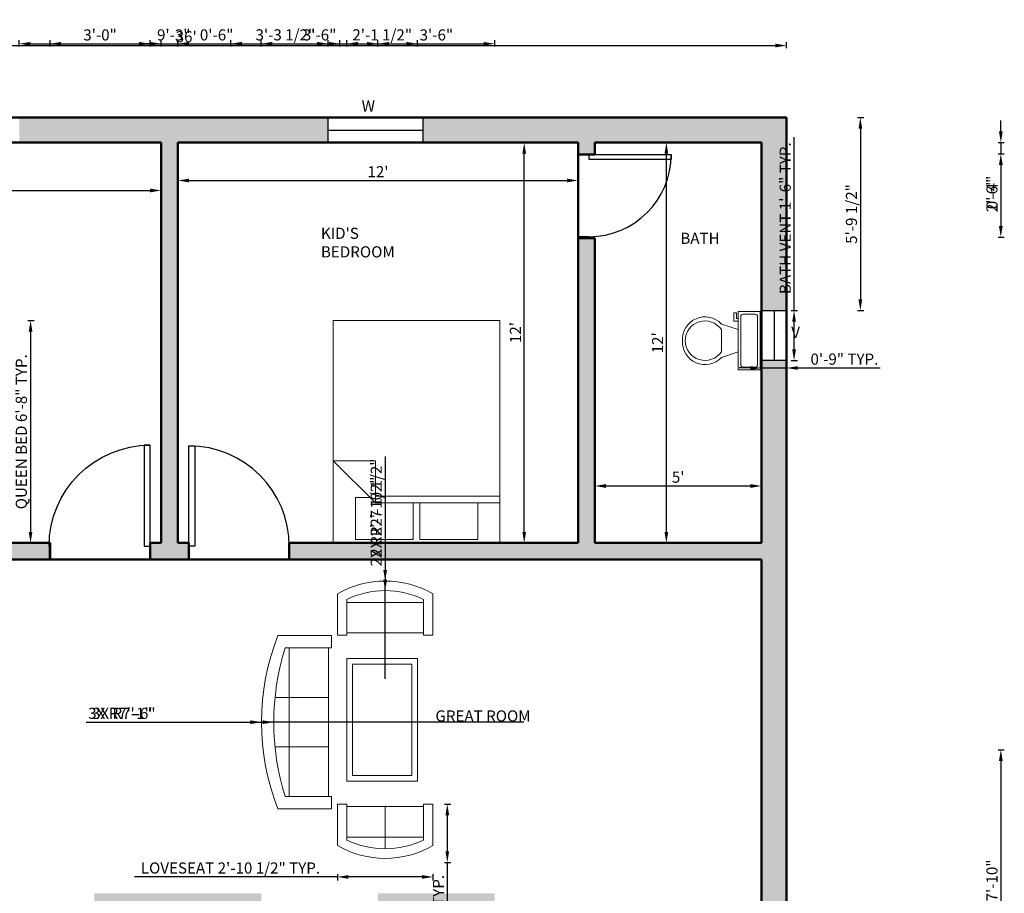
# Model space of a CAD drawing. Units: inches. Extents: x -31 to 511, y -453 to 49.
# Tile 4 of 4: x 157 to 511, y -265 to 49. Entities that reach past the tile are written whole.
import ezdxf

# ---------------------------------------------------------------- set-up
doc = ezdxf.new("R2010")
doc.units = ezdxf.units.IN
for name, color, linetype, lineweight in [('A-ANNO-DIMS', 2, 'Continuous', 18), ('A-ANNO-TEXT', 7, 'Continuous', 18), ('A-AREA-IDEN', 7, 'Continuous', 25), ('A-DOOR', 3, 'Continuous', 25), ('A-FLOR-FIXT', 9, 'Continuous', 18), ('A-FURN', 8, 'Continuous', 18), ('A-GLAZ', 4, 'Continuous', 25), ('A-WALL', 7, 'Continuous', 50), ('A-WALL-PATT', 252, 'Continuous', 13)]:
    doc.layers.add(name, color=color, linetype=linetype, lineweight=lineweight)
doc.styles.get("Standard").update_dxf_attribs({"font": 'arial.ttf'})
doc.dimstyles.new('ISO-25', dxfattribs={"dimtxt": 4, "dimasz": 4, "dimexe": 1.25, "dimexo": 0.625, "dimtad": 1, "dimlunit": 3, "dimtxsty": 'Standard', "dimcen": 2.5, "dimadec": 0, "dimazin": 0, "dimtfac": 1, "dimtmove": 0, "dimatfit": 3, "dimfxl": 1, "dimfxlon": 1, "dimarcsym": 0})

# ---------------------------------------------------------------- blocks, each defined once
blk = doc.blocks.new('*U2')
for p, q in [((0, 0), (0, -100)), ((750, 0), (750, -100))]:
    blk.add_line(p, q)
blk.add_lwpolyline([(0, 0), (0, 750), (43.75, 750), (43.75, 0)], close=True)
blk.add_arc((0, 0), 750, 0, 90)
blk = doc.blocks.new('*U4')
for p, q in [((9.5, -6), (9.5, -2)), ((-10, -8.5), (-8, -8.5)), ((-10, -9.5), (-10, -8.5)), ((-7, -9.5), (-10, -9.5)), ((-8, -8.5), (-8, -8)), ((-7, -8), (-7, -9.5)), ((-4, -8), (-6, -14)), ((4, -8), (6, -14)), ((4, -14), (-4, -14))]:
    blk.add_line(p, q)
blk.add_lwpolyline([(10.5, -8), (10.5, 0), (-10.5, 0), (-10.5, -8)], close=True)
for points in [[(-9.5, -2), (-9.5, -6)], [(8.5, -1), (-8.5, -1)], [(-8.5, -7), (8.5, -7)]]:
    blk.add_lwpolyline(points)
for centre, radius, start, end in [((-8.625, -1.875), 0.8839, 81.8699, 188.1301), ((8.625, -1.875), 0.8839, 351.8699, 98.1301), ((-8.625, -6.125), 0.8839, 171.869898, 278.1301), ((8.625, -6.125), 0.8839, 261.8699, 8.1301), ((-0.4772, -19.9188), 8.0953, 133.01722, 273.38), ((0.0374, -19.8731), 7.127, 124.50543, 269.7), ((-0.0373, -19.8731), 7.127, 270.3, 55.4946), ((0.4773, -19.9188), 8.0953, 266.62, 46.9828)]:
    blk.add_arc(centre, radius, start, end)
blk = doc.blocks.new('Sofa - Roundback Loveseat 5 ft.')
for p, q in [((0, -32.44198), (0, -5.99998)), ((-24, -33.99998), (-24, -11.46958)), ((24.00004, -33.99998), (24.00004, -11.46958)), ((-23.9998, -13.38178), (23.99986, -13.38178)), ((-24, -32.44198), (24.00004, -32.44198))]:
    blk.add_line(p, q)
for points in [[(-24, -33.99998), (-30, -33.99998), (-30, -7.99998)], [(30.00004, -7.99998), (30.00004, -33.99998), (24.00004, -33.99998)]]:
    blk.add_lwpolyline(points)
for centre, radius, start, end in [((0, -60.24998), 60.24998, 60.13715, 119.8628), ((0, -61.38438), 55.38444, 64.32083, 115.6792)]:
    blk.add_arc(centre, radius, start, end)
blk = doc.blocks.new('Bed - Queen')
for p, q in [((0, -80.00003), (0, 0)), ((0, 0), (59.99999, 0)), ((59.99999, 0), (59.99999, -80.00003)), ((7.99999, -1.2), (28.79998, -1.2)), ((7.99999, -14.4), (7.99999, -1.2)), ((28.79998, -1.2), (28.79998, -14.4)), ((31.19999, -1.2), (51.99999, -1.2)), ((31.19999, -14.4), (31.19999, -1.2)), ((51.99999, -1.2), (51.99999, -16.4)), ((0, -14.4), (44.8, -14.4)), ((44.8, -16.8), (0, -16.8)), ((59.99999, -29.6), (44.8, -14.4)), ((44.8, -14.4), (44.8, -29.6)), ((51.99999, -16.4), (46.79936, -16.4)), ((44.8, -29.6), (59.99999, -29.6)), ((59.99999, -80.00003), (0, -80.00003))]:
    blk.add_line(p, q)
blk = doc.blocks.new('Sofa - Roundback 7 ft.')
for p, q in [((-12.00002, -32.4421), (-12.00003, -6.5971)), ((11.99997, -32.4421), (11.99998, -6.5971)), ((-36.000027, -34), (-36.000027, -11.4696)), ((-35.999844, -13.3819), (35.9998, -13.3819)), ((35.99998, -34), (35.99998, -11.4696)), ((-36.000027, -32.4421), (35.99998, -32.4421))]:
    blk.add_line(p, q)
for points in [[(-36.000027, -34), (-42.000027, -34), (-42.000027, -8)], [(41.99998, -8), (41.99998, -34), (35.99998, -34)]]:
    blk.add_lwpolyline(points)
for centre, radius, start, end in [((0, -114.25), 114.25, 68.43141, 111.5686), ((-0.00001, -127.1968), 121.1968, 72.72033, 107.2797)]:
    blk.add_arc(centre, radius, start, end)
blk = doc.blocks.new('*D14')
at = {"layer": 'A-ANNO-DIMS', "color": 0, "lineweight": -2, "transparency": 16777216}
for p, q in [((63.46, -11.59), (63.46, -13.84)), ((67.46, -12.59), (203.46, -12.59)), ((207.46, -11.59), (207.46, -13.84))]:
    blk.add_line(p, q, dxfattribs=at)
at = {"layer": 'A-ANNO-DIMS', "color": 0, "transparency": 16777216}
for points in [[(67.46, -11.92), (67.46, -13.25), (63.46, -12.59)], [(203.46, -11.92), (203.46, -13.25), (207.46, -12.59)]]:
    blk.add_solid(points, dxfattribs=at)
at = {"layer": 'Defpoints', "color": 0, "transparency": 16777216}
for p in [(63.46, 4.62), (207.46, 4.62), (207.46, -12.59)]:
    blk.add_point(p, dxfattribs=at)
at = {"layer": 'A-ANNO-DIMS', "color": 0, "transparency": 16777216, "insert": (135.46, -9.95), "char_height": 4, "attachment_point": 5}
blk.add_mtext("12'", dxfattribs=at)
blk = doc.blocks.new('*D16')
at = {"layer": 'A-ANNO-DIMS', "color": 0, "lineweight": -2, "transparency": 16777216}
for p, q in [((213.46, -8.01), (213.46, -10.26)), ((217.46, -9.01), (353.46, -9.01)), ((357.46, -8.01), (357.46, -10.26))]:
    blk.add_line(p, q, dxfattribs=at)
at = {"layer": 'A-ANNO-DIMS', "color": 0, "transparency": 16777216}
for points in [[(217.46, -8.34), (217.46, -9.67), (213.46, -9.01)], [(353.46, -8.34), (353.46, -9.67), (357.46, -9.01)]]:
    blk.add_solid(points, dxfattribs=at)
at = {"layer": 'Defpoints', "color": 0, "transparency": 16777216}
for p in [(213.46, 4.62), (357.46, 4.62), (357.46, -9.01)]:
    blk.add_point(p, dxfattribs=at)
at = {"layer": 'A-ANNO-DIMS', "color": 0, "transparency": 16777216, "insert": (285.46, -6.37), "char_height": 4, "attachment_point": 5}
blk.add_mtext("12'", dxfattribs=at)
blk = doc.blocks.new('*D17')
at = {"layer": 'A-ANNO-DIMS', "color": 0, "lineweight": -2, "transparency": 16777216}
for p, q in [((339.07, 4.62), (336.82, 4.62)), ((338.07, -135.38), (338.07, 0.62)), ((339.07, -139.38), (336.82, -139.38))]:
    blk.add_line(p, q, dxfattribs=at)
at = {"layer": 'A-ANNO-DIMS', "color": 0, "transparency": 16777216}
for points in [[(337.4, 0.62), (338.73, 0.62), (338.07, 4.62)], [(337.4, -135.38), (338.73, -135.38), (338.07, -139.38)]]:
    blk.add_solid(points, dxfattribs=at)
at = {"layer": 'Defpoints', "color": 0, "transparency": 16777216}
for p in [(338.07, 4.62), (357.46, 4.62), (357.46, -139.38)]:
    blk.add_point(p, dxfattribs=at)
at = {"layer": 'A-ANNO-DIMS', "color": 0, "transparency": 16777216, "insert": (335.43, -63.69), "char_height": 4, "attachment_point": 5, "rotation": 90}
blk.add_mtext("12'", dxfattribs=at)
blk = doc.blocks.new('*D18')
at = {"layer": 'A-ANNO-DIMS', "color": 0, "lineweight": -2, "transparency": 16777216}
for p, q in [((363.46, -119.88), (363.46, -117.63)), ((367.46, -118.88), (419.46, -118.88)), ((423.46, -119.88), (423.46, -117.63))]:
    blk.add_line(p, q, dxfattribs=at)
at = {"layer": 'A-ANNO-DIMS', "color": 0, "transparency": 16777216}
for points in [[(367.46, -118.21), (367.46, -119.55), (363.46, -118.88)], [(419.46, -118.21), (419.46, -119.55), (423.46, -118.88)]]:
    blk.add_solid(points, dxfattribs=at)
at = {"layer": 'Defpoints', "color": 0, "transparency": 16777216}
for p in [(423.46, -118.88), (363.46, -139.38), (423.46, -139.38)]:
    blk.add_point(p, dxfattribs=at)
at = {"layer": 'A-ANNO-DIMS', "color": 0, "transparency": 16777216, "insert": (393.46, -116.22), "char_height": 4, "attachment_point": 5}
blk.add_mtext("5'", dxfattribs=at)
blk = doc.blocks.new('*D19')
at = {"layer": 'A-ANNO-DIMS', "color": 0, "lineweight": -2, "transparency": 16777216}
for p, q in [((390.21, 4.62), (387.96, 4.62)), ((389.21, -135.38), (389.21, 0.62)), ((390.21, -139.38), (387.96, -139.38))]:
    blk.add_line(p, q, dxfattribs=at)
at = {"layer": 'A-ANNO-DIMS', "color": 0, "transparency": 16777216}
for points in [[(388.54, 0.62), (389.88, 0.62), (389.21, 4.62)], [(388.54, -135.38), (389.88, -135.38), (389.21, -139.38)]]:
    blk.add_solid(points, dxfattribs=at)
at = {"layer": 'Defpoints', "color": 0, "transparency": 16777216}
for p in [(389.21, 4.62), (423.46, 4.62), (423.46, -139.38)]:
    blk.add_point(p, dxfattribs=at)
at = {"layer": 'A-ANNO-DIMS', "color": 0, "transparency": 16777216, "insert": (386.58, -67.38), "char_height": 4, "attachment_point": 5, "rotation": 90}
blk.add_mtext("12'", dxfattribs=at)
blk = doc.blocks.new('*D26')
at = {"layer": 'A-ANNO-DIMS', "color": 0, "lineweight": -2, "transparency": 16777216}
for p, q in [((0.46, 38.54), (0.46, 40.79)), ((4.46, 39.54), (428.46, 39.54)), ((432.46, 38.54), (432.46, 40.79))]:
    blk.add_line(p, q, dxfattribs=at)
at = {"layer": 'A-ANNO-DIMS', "color": 0, "transparency": 16777216}
for points in [[(4.46, 40.2), (4.46, 38.87), (0.46, 39.54)], [(428.46, 40.2), (428.46, 38.87), (432.46, 39.54)]]:
    blk.add_solid(points, dxfattribs=at)
at = {"layer": 'Defpoints', "color": 0, "transparency": 16777216}
for p in [(432.46, 39.54), (0.46, 13.62), (432.46, 13.62)]:
    blk.add_point(p, dxfattribs=at)
at = {"layer": 'A-ANNO-DIMS', "color": 0, "transparency": 16777216, "insert": (216.46, 42.21), "char_height": 4, "attachment_point": 5}
blk.add_mtext("36'", dxfattribs=at)
blk = doc.blocks.new('WIN-34IN')
blk.add_line((0, 4.5), (34, 4.5))
blk.add_lwpolyline([(0, 9), (34, 9), (34, 0), (0, 0)], close=True)
blk = doc.blocks.new('VENT-18IN')
blk.add_line((4.5, 18), (4.5, 0))
blk.add_lwpolyline([(0, 18), (9, 18), (9, 0), (0, 0)], close=True)
blk = doc.blocks.new('*D32')
at = {"layer": 'A-ANNO-DIMS', "color": 0, "lineweight": -2, "transparency": 16777216}
for p, q in [((435.16, -55.74), (435.16, 6.62)), ((434.16, -55.74), (436.41, -55.74)), ((435.16, -69.74), (435.16, -59.74)), ((434.16, -73.74), (436.41, -73.74))]:
    blk.add_line(p, q, dxfattribs=at)
at = {"layer": 'A-ANNO-DIMS', "color": 0, "transparency": 16777216}
for points in [[(434.5, -59.74), (435.83, -59.74), (435.16, -55.74)], [(434.5, -69.74), (435.83, -69.74), (435.16, -73.74)]]:
    blk.add_solid(points, dxfattribs=at)
at = {"layer": 'Defpoints', "color": 0, "transparency": 16777216}
for p in [(432.46, -55.74), (435.16, -55.74), (432.46, -73.74)]:
    blk.add_point(p, dxfattribs=at)
at = {"layer": 'A-ANNO-DIMS', "color": 0, "transparency": 16777216, "insert": (432.5, -22.56), "char_height": 4, "attachment_point": 5, "rotation": 90}
blk.add_mtext('BATH VENT 1\'-6" TYP.', dxfattribs=at)
blk = doc.blocks.new('*D33')
at = {"layer": 'A-ANNO-DIMS', "color": 0, "lineweight": -2, "transparency": 16777216}
for p, q in [((419.46, -76.44), (415.46, -76.44)), ((423.46, -75.44), (423.46, -77.69)), ((423.46, -76.44), (432.46, -76.44)), ((432.46, -75.44), (432.46, -77.69)), ((436.46, -76.44), (466.1, -76.44))]:
    blk.add_line(p, q, dxfattribs=at)
at = {"layer": 'A-ANNO-DIMS', "color": 0, "transparency": 16777216}
for points in [[(419.46, -75.78), (419.46, -77.11), (423.46, -76.44)], [(436.46, -75.78), (436.46, -77.11), (432.46, -76.44)]]:
    blk.add_solid(points, dxfattribs=at)
at = {"layer": 'Defpoints', "color": 0, "transparency": 16777216}
for p in [(423.46, -73.74), (432.46, -73.74), (432.46, -76.44)]:
    blk.add_point(p, dxfattribs=at)
at = {"layer": 'A-ANNO-DIMS', "color": 0, "transparency": 16777216, "insert": (453.28, -73.77), "char_height": 4, "attachment_point": 5}
blk.add_mtext('0\'-9" TYP.', dxfattribs=at)
blk = doc.blocks.new('*D34')
at = {"layer": 'A-ANNO-DIMS', "color": 0, "lineweight": -2, "transparency": 16777216}
for p, q in [((159.47, -59.38), (161.72, -59.38)), ((160.47, -63.38), (160.47, -135.38)), ((159.47, -139.38), (161.72, -139.38))]:
    blk.add_line(p, q, dxfattribs=at)
at = {"layer": 'A-ANNO-DIMS', "color": 0, "transparency": 16777216}
for points in [[(159.8, -63.38), (161.13, -63.38), (160.47, -59.38)], [(159.8, -135.38), (161.13, -135.38), (160.47, -139.38)]]:
    blk.add_solid(points, dxfattribs=at)
at = {"layer": 'Defpoints', "color": 0, "transparency": 16777216}
for p in [(148.47, -59.38), (148.47, -139.38), (160.47, -139.38)]:
    blk.add_point(p, dxfattribs=at)
at = {"layer": 'A-ANNO-DIMS', "color": 0, "transparency": 16777216, "insert": (157.65, -99.38), "char_height": 4, "attachment_point": 5, "rotation": 90}
blk.add_mtext('QUEEN BED 6\'-8" TYP.', dxfattribs=at)
blk = doc.blocks.new('*D38')
at = {"layer": 'A-ANNO-DIMS', "color": 0, "lineweight": -2, "transparency": 16777216}
for p, q in [((270.85, -258.5), (270.85, -260.75)), ((305.24, -258.5), (305.24, -260.75)), ((270.85, -259.5), (197.91, -259.5)), ((301.24, -259.5), (274.85, -259.5))]:
    blk.add_line(p, q, dxfattribs=at)
at = {"layer": 'A-ANNO-DIMS', "color": 0, "transparency": 16777216}
for points in [[(274.85, -258.83), (274.85, -260.17), (270.85, -259.5)], [(301.24, -258.83), (301.24, -260.17), (305.24, -259.5)]]:
    blk.add_solid(points, dxfattribs=at)
at = {"layer": 'Defpoints', "color": 0, "transparency": 16777216}
for p in [(270.85, -254.34), (305.24, -254.34), (270.85, -259.5)]:
    blk.add_point(p, dxfattribs=at)
at = {"layer": 'A-ANNO-DIMS', "color": 0, "transparency": 16777216, "insert": (232.38, -256.8), "char_height": 4, "attachment_point": 5}
blk.add_mtext('LOVESEAT 2\'-10 1/2" TYP.', dxfattribs=at)
blk = doc.blocks.new('*D39')
at = {"layer": 'A-ANNO-DIMS', "color": 0, "lineweight": -2, "transparency": 16777216}
for p, q in [((309.4, -233.32), (311.65, -233.32)), ((310.4, -237.32), (310.4, -250.34)), ((309.4, -254.34), (311.65, -254.34)), ((310.4, -254.34), (310.4, -283.6))]:
    blk.add_line(p, q, dxfattribs=at)
at = {"layer": 'A-ANNO-DIMS', "color": 0, "transparency": 16777216}
for points in [[(309.73, -237.32), (311.06, -237.32), (310.4, -233.32)], [(309.73, -250.34), (311.06, -250.34), (310.4, -254.34)]]:
    blk.add_solid(points, dxfattribs=at)
at = {"layer": 'Defpoints', "color": 0, "transparency": 16777216}
for p in [(305.24, -233.32), (305.24, -254.34), (310.4, -254.34)]:
    blk.add_point(p, dxfattribs=at)
at = {"layer": 'A-ANNO-DIMS', "color": 0, "transparency": 16777216, "insert": (307.73, -270.97), "char_height": 4, "attachment_point": 5, "rotation": 90}
blk.add_mtext('1\'-9" TYP.', dxfattribs=at)
blk = doc.blocks.new('*D50')
at = {"layer": 'A-ANNO-DIMS', "color": 0, "lineweight": -2, "transparency": 16777216}
for p, q in [((167.46, 39.17), (167.46, 41.42)), ((171.46, 40.17), (199.46, 40.17)), ((203.46, 39.17), (203.46, 41.42))]:
    blk.add_line(p, q, dxfattribs=at)
at = {"layer": 'A-ANNO-DIMS', "color": 0, "transparency": 16777216}
for points in [[(171.46, 40.84), (171.46, 39.5), (167.46, 40.17)], [(199.46, 40.84), (199.46, 39.5), (203.46, 40.17)]]:
    blk.add_solid(points, dxfattribs=at)
at = {"layer": 'Defpoints', "color": 0, "transparency": 16777216}
for p in [(203.46, 40.17), (167.46, -139.38), (203.46, -139.38)]:
    blk.add_point(p, dxfattribs=at)
at = {"layer": 'A-ANNO-DIMS', "color": 0, "transparency": 16777216, "insert": (185.46, 42.84), "char_height": 4, "attachment_point": 5}
blk.add_mtext('3\'-0"', dxfattribs=at)
blk = doc.blocks.new('*D51')
at = {"layer": 'A-ANNO-DIMS', "color": 0, "lineweight": -2, "transparency": 16777216}
for p, q in [((508.55, 0.62), (510.8, 0.62)), ((509.55, -3.38), (509.55, -25.38)), ((508.55, -29.38), (510.8, -29.38))]:
    blk.add_line(p, q, dxfattribs=at)
at = {"layer": 'A-ANNO-DIMS', "color": 0, "transparency": 16777216}
for points in [[(508.88, -3.38), (510.22, -3.38), (509.55, 0.62)], [(508.88, -25.38), (510.22, -25.38), (509.55, -29.38)]]:
    blk.add_solid(points, dxfattribs=at)
at = {"layer": 'Defpoints', "color": 0, "transparency": 16777216}
for p in [(57.46, 0.62), (57.46, -29.38), (509.55, -29.38)]:
    blk.add_point(p, dxfattribs=at)
at = {"layer": 'A-ANNO-DIMS', "color": 0, "transparency": 16777216, "insert": (506.88, -14.38), "char_height": 4, "attachment_point": 5, "rotation": 90}
blk.add_mtext('2\'-6"', dxfattribs=at)
blk = doc.blocks.new('*D52')
at = {"layer": 'A-ANNO-DIMS', "color": 0, "lineweight": -2, "transparency": 16777216}
for p, q in [((243.45, 39.17), (243.45, 41.42)), ((247.45, 40.17), (281.45, 40.17)), ((285.45, 39.17), (285.45, 41.42))]:
    blk.add_line(p, q, dxfattribs=at)
at = {"layer": 'A-ANNO-DIMS', "color": 0, "transparency": 16777216}
for points in [[(247.45, 40.84), (247.45, 39.5), (243.45, 40.17)], [(281.45, 40.84), (281.45, 39.5), (285.45, 40.17)]]:
    blk.add_solid(points, dxfattribs=at)
at = {"layer": 'Defpoints', "color": 0, "transparency": 16777216}
for p in [(285.45, 40.17), (243.45, -265.38), (285.45, -265.38)]:
    blk.add_point(p, dxfattribs=at)
at = {"layer": 'A-ANNO-DIMS', "color": 0, "transparency": 16777216, "insert": (264.45, 42.84), "char_height": 4, "attachment_point": 5}
blk.add_mtext('3\'-6"', dxfattribs=at)
blk = doc.blocks.new('*D53')
at = {"layer": 'A-ANNO-DIMS', "color": 0, "lineweight": -2, "transparency": 16777216}
for p, q in [((203.46, 40.17), (199.46, 40.17)), ((207.46, 39.17), (207.46, 41.42)), ((207.46, 40.17), (213.46, 40.17)), ((213.46, 39.17), (213.46, 41.42)), ((217.46, 40.17), (233.35, 40.17))]:
    blk.add_line(p, q, dxfattribs=at)
at = {"layer": 'A-ANNO-DIMS', "color": 0, "transparency": 16777216}
for points in [[(203.46, 40.84), (203.46, 39.5), (207.46, 40.17)], [(217.46, 40.84), (217.46, 39.5), (213.46, 40.17)]]:
    blk.add_solid(points, dxfattribs=at)
at = {"layer": 'Defpoints', "color": 0, "transparency": 16777216}
for p in [(213.46, 40.17), (207.46, 4.62), (213.46, 4.62)]:
    blk.add_point(p, dxfattribs=at)
at = {"layer": 'A-ANNO-DIMS', "color": 0, "transparency": 16777216, "insert": (227.41, 42.84), "char_height": 4, "attachment_point": 5}
blk.add_mtext('0\'-6"', dxfattribs=at)
blk = doc.blocks.new('*D55')
at = {"layer": 'A-ANNO-DIMS', "color": 0, "lineweight": -2, "transparency": 16777216}
for p, q in [((156.41, 39.17), (156.41, 41.42)), ((160.41, 40.17), (263.57, 40.17)), ((267.57, 39.17), (267.57, 41.42))]:
    blk.add_line(p, q, dxfattribs=at)
at = {"layer": 'A-ANNO-DIMS', "color": 0, "transparency": 16777216}
for points in [[(160.41, 40.84), (160.41, 39.5), (156.41, 40.17)], [(263.57, 40.84), (263.57, 39.5), (267.57, 40.17)]]:
    blk.add_solid(points, dxfattribs=at)
at = {"layer": 'Defpoints', "color": 0, "transparency": 16777216}
for p in [(267.57, 40.17), (156.41, 13.62), (267.57, 13.62)]:
    blk.add_point(p, dxfattribs=at)
at = {"layer": 'A-ANNO-DIMS', "color": 0, "transparency": 16777216, "insert": (211.99, 42.84), "char_height": 4, "attachment_point": 5}
blk.add_mtext('9\'-3"', dxfattribs=at)
blk = doc.blocks.new('*D56')
at = {"layer": 'A-ANNO-DIMS', "color": 0, "lineweight": -2, "transparency": 16777216}
for p, q in [((458.01, 13.62), (460.26, 13.62)), ((459.01, 9.62), (459.01, -51.74)), ((458.01, -55.74), (460.26, -55.74))]:
    blk.add_line(p, q, dxfattribs=at)
at = {"layer": 'A-ANNO-DIMS', "color": 0, "transparency": 16777216}
for points in [[(458.35, 9.62), (459.68, 9.62), (459.01, 13.62)], [(458.35, -51.74), (459.68, -51.74), (459.01, -55.74)]]:
    blk.add_solid(points, dxfattribs=at)
at = {"layer": 'Defpoints', "color": 0, "transparency": 16777216}
for p in [(432.46, 13.62), (432.46, -55.74), (459.01, -55.74)]:
    blk.add_point(p, dxfattribs=at)
at = {"layer": 'A-ANNO-DIMS', "color": 0, "transparency": 16777216, "insert": (456.32, -21.06), "char_height": 4, "attachment_point": 5, "rotation": 90}
blk.add_mtext('5\'-9 1/2"', dxfattribs=at)
blk = doc.blocks.new('*D58')
at = {"layer": 'A-ANNO-DIMS', "color": 0, "lineweight": -2, "transparency": 16777216}
for p, q in [((508.55, -213.76), (510.8, -213.76)), ((509.55, -217.76), (509.55, -303.74)), ((508.55, -307.74), (510.8, -307.74))]:
    blk.add_line(p, q, dxfattribs=at)
at = {"layer": 'A-ANNO-DIMS', "color": 0, "transparency": 16777216}
for points in [[(508.88, -217.76), (510.22, -217.76), (509.55, -213.76)], [(508.88, -303.74), (510.22, -303.74), (509.55, -307.74)]]:
    blk.add_solid(points, dxfattribs=at)
at = {"layer": 'Defpoints', "color": 0, "transparency": 16777216}
for p in [(9.46, -213.76), (9.46, -307.74), (509.55, -307.74)]:
    blk.add_point(p, dxfattribs=at)
at = {"layer": 'A-ANNO-DIMS', "color": 0, "transparency": 16777216, "insert": (506.88, -260.75), "char_height": 4, "attachment_point": 5, "rotation": 90}
blk.add_mtext('7\'-10"', dxfattribs=at)
blk = doc.blocks.new('*D63')
at = {"layer": 'A-ANNO-DIMS', "color": 0, "lineweight": -2, "transparency": 16777216}
for p, q in [((285.45, 39.17), (285.45, 41.42)), ((289.45, 40.17), (323.46, 40.17)), ((327.46, 39.17), (327.46, 41.42))]:
    blk.add_line(p, q, dxfattribs=at)
at = {"layer": 'A-ANNO-DIMS', "color": 0, "transparency": 16777216}
for points in [[(289.45, 40.84), (289.45, 39.5), (285.45, 40.17)], [(323.46, 40.84), (323.46, 39.5), (327.46, 40.17)]]:
    blk.add_solid(points, dxfattribs=at)
at = {"layer": 'Defpoints', "color": 0, "transparency": 16777216}
for p in [(327.46, 40.17), (285.45, -265.38), (327.46, -265.38)]:
    blk.add_point(p, dxfattribs=at)
at = {"layer": 'A-ANNO-DIMS', "color": 0, "transparency": 16777216, "insert": (306.46, 42.84), "char_height": 4, "attachment_point": 5}
blk.add_mtext('3\'-6"', dxfattribs=at)
blk = doc.blocks.new('*D67')
at = {"layer": 'A-ANNO-DIMS', "color": 0, "lineweight": -2, "transparency": 16777216}
for p, q in [((274.24, 39.17), (274.24, 41.42)), ((278.24, 40.17), (295.69, 40.17)), ((299.69, 39.17), (299.69, 41.42))]:
    blk.add_line(p, q, dxfattribs=at)
at = {"layer": 'A-ANNO-DIMS', "color": 0, "transparency": 16777216}
for points in [[(278.24, 40.84), (278.24, 39.5), (274.24, 40.17)], [(295.69, 40.84), (295.69, 39.5), (299.69, 40.17)]]:
    blk.add_solid(points, dxfattribs=at)
at = {"layer": 'Defpoints', "color": 0, "transparency": 16777216}
for p in [(299.69, 40.17), (274.24, -180.94), (299.69, -180.94)]:
    blk.add_point(p, dxfattribs=at)
at = {"layer": 'A-ANNO-DIMS', "color": 0, "transparency": 16777216, "insert": (286.97, 42.86), "char_height": 4, "attachment_point": 5}
blk.add_mtext('2\'-1 1/2"', dxfattribs=at)
blk = doc.blocks.new('*D68')
at = {"layer": 'A-ANNO-DIMS', "color": 0, "lineweight": -2, "transparency": 16777216}
for p, q in [((-25.09, -180.94), (-27.34, -180.94)), ((-26.09, -221.03), (-26.09, -184.94)), ((-25.09, -225.03), (-27.34, -225.03))]:
    blk.add_line(p, q, dxfattribs=at)
at = {"layer": 'A-ANNO-DIMS', "color": 0, "transparency": 16777216}
for points in [[(-26.75, -184.94), (-25.42, -184.94), (-26.09, -180.94)], [(-26.75, -221.03), (-25.42, -221.03), (-26.09, -225.03)]]:
    blk.add_solid(points, dxfattribs=at)
at = {"layer": 'Defpoints', "color": 0, "transparency": 16777216}
for p in [(-26.09, -180.94), (299.69, -180.94), (299.69, -225.03)]:
    blk.add_point(p, dxfattribs=at)
at = {"layer": 'A-ANNO-DIMS', "color": 0, "transparency": 16777216, "insert": (-28.75, -202.99), "char_height": 4, "attachment_point": 5, "rotation": 90}
blk.add_mtext('3\'-8"', dxfattribs=at)
blk = doc.blocks.new('*D69')
at = {"layer": 'A-ANNO-DIMS', "color": 0, "lineweight": -2, "transparency": 16777216}
for p, q in [((232.48, 39.17), (232.48, 41.42)), ((236.48, 40.17), (267.79, 40.17)), ((271.79, 39.17), (271.79, 41.42))]:
    blk.add_line(p, q, dxfattribs=at)
at = {"layer": 'A-ANNO-DIMS', "color": 0, "transparency": 16777216}
for points in [[(236.48, 40.84), (236.48, 39.5), (232.48, 40.17)], [(267.79, 40.84), (267.79, 39.5), (271.79, 40.17)]]:
    blk.add_solid(points, dxfattribs=at)
at = {"layer": 'Defpoints', "color": 0, "transparency": 16777216}
for p in [(271.79, 40.17), (232.48, -304.06), (271.79, -304.06)]:
    blk.add_point(p, dxfattribs=at)
at = {"layer": 'A-ANNO-DIMS', "color": 0, "transparency": 16777216, "insert": (252.13, 42.86), "char_height": 4, "attachment_point": 5}
blk.add_mtext('3\'-3 1/2"', dxfattribs=at)
blk = doc.blocks.new('*D71')
at = {"layer": 'A-ANNO-DIMS', "color": 0, "lineweight": -2, "transparency": 16777216}
for p, q in [((209.46, -444.93), (205.46, -444.93)), ((213.46, -443.93), (213.46, -446.18)), ((213.46, -444.93), (217.46, -444.93)), ((217.46, -443.93), (217.46, -446.18)), ((221.46, -444.93), (237.35, -444.93))]:
    blk.add_line(p, q, dxfattribs=at)
at = {"layer": 'A-ANNO-DIMS', "color": 0, "transparency": 16777216}
for points in [[(209.46, -444.26), (209.46, -445.6), (213.46, -444.93)], [(221.46, -444.26), (221.46, -445.6), (217.46, -444.93)]]:
    blk.add_solid(points, dxfattribs=at)
at = {"layer": 'Defpoints', "color": 0, "transparency": 16777216}
for p in [(213.46, -139.38), (217.46, -139.38), (217.46, -444.93)]:
    blk.add_point(p, dxfattribs=at)
at = {"layer": 'A-ANNO-DIMS', "color": 0, "transparency": 16777216, "insert": (231.41, -442.26), "char_height": 4, "attachment_point": 5}
blk.add_mtext('0\'-4"', dxfattribs=at)
blk = doc.blocks.new('*D72')
at = {"layer": 'A-ANNO-DIMS', "color": 0, "lineweight": -2, "transparency": 16777216}
for p, q in [((509.55, 8.62), (509.55, 12.62)), ((508.55, 4.62), (510.8, 4.62)), ((509.55, 4.62), (509.55, 0.62)), ((508.55, 0.62), (510.8, 0.62)), ((509.55, -3.38), (509.55, -19.26))]:
    blk.add_line(p, q, dxfattribs=at)
at = {"layer": 'A-ANNO-DIMS', "color": 0, "transparency": 16777216}
for points in [[(508.88, 8.62), (510.22, 8.62), (509.55, 4.62)], [(508.88, -3.38), (510.22, -3.38), (509.55, 0.62)]]:
    blk.add_solid(points, dxfattribs=at)
at = {"layer": 'Defpoints', "color": 0, "transparency": 16777216}
for p in [(57.46, 4.62), (57.46, 0.62), (509.55, 0.62)]:
    blk.add_point(p, dxfattribs=at)
at = {"layer": 'A-ANNO-DIMS', "color": 0, "transparency": 16777216, "insert": (506.88, -13.32), "char_height": 4, "attachment_point": 5, "rotation": 90}
blk.add_mtext('0\'-4"', dxfattribs=at)
blk = doc.blocks.new('*D73')
at = {"layer": 'A-ANNO-DIMS', "color": 0, "lineweight": -2, "transparency": 16777216}
for p, q in [((181.83, -203.84), (243.98, -203.84)), ((337.97, -203.84), (247.98, -203.84))]:
    blk.add_line(p, q, dxfattribs=at)
at = {"layer": 'A-ANNO-DIMS', "color": 0, "transparency": 16777216}
blk.add_solid([(243.98, -203.17), (243.98, -204.51), (247.98, -203.84)], dxfattribs=at)
at = {"layer": 'Defpoints', "color": 0, "transparency": 16777216}
for p in [(247.98, -203.84), (337.97, -203.84)]:
    blk.add_point(p, dxfattribs=at)
at = {"layer": 'A-ANNO-DIMS', "color": 0, "transparency": 16777216, "insert": (193.99, -201.17), "char_height": 4, "attachment_point": 5, "rotation": 359.9999}
blk.add_mtext('3X R7\'-6"', dxfattribs=at)
blk = doc.blocks.new('*D74')
at = {"layer": 'A-ANNO-DIMS', "color": 0, "lineweight": -2, "transparency": 16777216}
for p, q in [((180.47, -203.84), (239.52, -203.84)), ((328.36, -203.84), (243.52, -203.84))]:
    blk.add_line(p, q, dxfattribs=at)
at = {"layer": 'A-ANNO-DIMS', "color": 0, "transparency": 16777216}
blk.add_solid([(239.52, -203.17), (239.52, -204.51), (243.52, -203.84)], dxfattribs=at)
at = {"layer": 'Defpoints', "color": 0, "transparency": 16777216}
for p in [(243.52, -203.84), (328.36, -203.84)]:
    blk.add_point(p, dxfattribs=at)
at = {"layer": 'A-ANNO-DIMS', "color": 0, "transparency": 16777216, "insert": (192.63, -201.17), "char_height": 4, "attachment_point": 5, "rotation": 359.9999}
blk.add_mtext('3X R7\'-1"', dxfattribs=at)
blk = doc.blocks.new('*D75')
at = {"layer": 'A-ANNO-DIMS', "color": 0, "lineweight": -2, "transparency": 16777216}
for p, q in [((288.04, -108.28), (288.04, -149.08)), ((288.04, -187.61), (288.04, -153.08))]:
    blk.add_line(p, q, dxfattribs=at)
at = {"layer": 'A-ANNO-DIMS', "color": 0, "transparency": 16777216}
blk.add_solid([(287.38, -149.08), (288.71, -149.08), (288.04, -153.08)], dxfattribs=at)
at = {"layer": 'Defpoints', "color": 0, "transparency": 16777216}
for p in [(288.04, -153.08), (288.04, -187.61)]:
    blk.add_point(p, dxfattribs=at)
at = {"layer": 'A-ANNO-DIMS', "color": 0, "transparency": 16777216, "insert": (285.35, -126.68), "char_height": 4, "attachment_point": 5, "rotation": 89.9992}
blk.add_mtext('2X R2\'-10 1/2"', dxfattribs=at)
blk = doc.blocks.new('*D76')
at = {"layer": 'A-ANNO-DIMS', "color": 0, "lineweight": -2, "transparency": 16777216}
for p, q in [((288.04, -114.83), (288.04, -152.52)), ((288.04, -188.26), (288.04, -156.52))]:
    blk.add_line(p, q, dxfattribs=at)
at = {"layer": 'A-ANNO-DIMS', "color": 0, "transparency": 16777216}
blk.add_solid([(287.38, -152.52), (288.71, -152.52), (288.04, -156.52)], dxfattribs=at)
at = {"layer": 'Defpoints', "color": 0, "transparency": 16777216}
for p in [(288.04, -156.52), (288.04, -188.26)]:
    blk.add_point(p, dxfattribs=at)
at = {"layer": 'A-ANNO-DIMS', "color": 0, "transparency": 16777216, "insert": (285.35, -131.67), "char_height": 4, "attachment_point": 5, "rotation": 89.9991}
blk.add_mtext('2X R2\'-7 1/2"', dxfattribs=at)

msp = doc.modelspace()

# ---------------------------------------------------------------- hatches: boundary and pattern name
at = {"layer": 'A-WALL-PATT'}
h = msp.add_hatch(color=256, dxfattribs=at)
h.dxf.hatch_style = 1
h.paths.add_polyline_path([(122.408, 13.62), (0.465, 13.62), (0.465, -55.742), (9.465, -55.742), (9.465, 4.62), (57.465, 4.62), (57.465, 0.62), (59.528, 0.62), (63.465, 0.62), (63.465, 4.62), (122.408, 4.62)])
h.paths.add_polyline_path([(267.569, 13.62), (156.408, 13.62), (156.408, 4.62), (207.465, 4.62), (207.465, -139.38), (203.465, -139.38), (203.465, -140.534), (203.465, -145.38), (217.465, -145.38), (217.465, -140.567), (217.465, -139.38), (213.465, -139.38), (213.465, 4.62), (267.569, 4.62)])
h.paths.add_polyline_path([(432.465, 13.62), (301.569, 13.62), (301.569, 4.62), (357.465, 4.62), (357.465, 0.312), (361.402, 0.312), (363.465, 0.312), (363.465, 4.62), (423.465, 4.62), (423.465, -55.742), (432.465, -55.742)])
h.paths.add_polyline_path([(432.465, -73.742), (423.465, -73.742), (423.465, -139.38), (363.465, -139.38), (363.465, -29.688), (357.465, -29.688), (357.465, -139.38), (253.542, -139.38, -0.0082235), (253.561, -140.567), (253.561, -145.38), (423.465, -145.38), (423.465, -409.38), (414.601, -409.38), (414.601, -412.759), (414.601, -418.38), (432.465, -418.38)])
h.paths.add_polyline_path([(167.12, -140.534, -0.00794), (167.139, -139.38), (63.465, -139.38), (63.465, -29.38), (57.465, -29.38), (57.465, -57.083), (57.472, -57.083), (57.472, -78.083), (57.465, -139.38), (9.465, -139.38), (9.465, -73.742), (0.465, -73.742), (0.465, -179.759), (9.465, -179.759), (9.465, -145.38), (167.12, -145.38)])
h.paths.add_polyline_path([(372.446, -412.759, -0.0200643), (372.581, -409.38), (327.465, -409.38), (327.465, -265.38), (285.454, -265.38), (285.454, -271.38), (321.465, -271.38), (321.465, -409.38), (273.096, -409.38), (273.096, -418.38), (372.446, -418.38)], flags=17)
h.paths.add_polyline_path([(239.096, -409.38), (189.465, -409.38), (189.465, -271.38), (243.454, -271.38), (243.454, -265.38), (183.465, -265.38), (183.465, -409.38), (156.552, -409.38), (156.552, -418.38), (239.096, -418.38)])
h.paths.add_polyline_path([(122.552, -409.38), (111.465, -409.38), (111.465, -325.38), (105.465, -325.38), (105.465, -409.38), (72.938, -409.38), (72.938, -418.38), (122.552, -418.38)])
h.paths.add_polyline_path([(38.938, -409.38), (9.465, -409.38), (9.465, -341.741), (0.465, -341.741), (0.465, -418.38), (38.938, -418.38)])
h.paths.add_polyline_path([(9.465, -213.759), (0.465, -213.759), (0.465, -307.741), (9.465, -307.741)])

# ---------------------------------------------------------------- linework, layer by layer
at = {"layer": 'A-FURN'}
for points in [[(274.239, -180.941), (299.695, -180.941), (299.695, -225.033), (274.239, -225.033)], [(276.239, -182.941), (297.695, -182.941), (297.695, -223.033), (276.239, -223.033)]]:
    msp.add_lwpolyline(points, close=True, dxfattribs=at)
at = {"layer": 'A-WALL'}
for p, q in [((0.465, 13.62), (432.465, 13.62)), ((432.465, 13.62), (432.465, -418.38)), ((63.465, 4.62), (207.465, 4.62)), ((207.465, -139.38), (207.465, 4.62)), ((213.465, 4.62), (357.465, 4.62)), ((213.465, -139.38), (213.465, 4.62)), ((357.465, -139.38), (357.465, 4.62)), ((363.465, 4.62), (423.465, 4.62)), ((363.465, 0.312), (363.465, 4.62)), ((423.465, 4.62), (423.465, -139.38)), ((363.465, 0.312), (357.465, 0.312)), ((363.465, -29.688), (357.465, -29.688)), ((363.465, -139.38), (363.465, -29.688)), ((63.465, -139.38), (167.465, -139.38)), ((167.465, -145.38), (167.465, -139.38)), ((203.465, -145.38), (203.465, -139.38)), ((203.465, -139.38), (207.465, -139.38)), ((213.465, -139.38), (217.465, -139.38)), ((217.465, -145.38), (217.465, -139.38)), ((253.465, -145.38), (253.465, -139.38)), ((253.465, -139.38), (357.465, -139.38)), ((363.465, -139.38), (423.465, -139.38)), ((9.465, -145.38), (423.465, -145.38)), ((423.465, -145.38), (423.465, -409.38))]:
    msp.add_line(p, q, dxfattribs=at)

# ---------------------------------------------------------------- block references
at = {"layer": 'A-DOOR', "xscale": 0.0393700787401575, "yscale": 0.0393700787401575, "zscale": 0.0393700787401575, "rotation": 270}
msp.add_blockref('*U2', (361.402, 0.312), dxfattribs=at)
at = {"layer": 'A-DOOR'}
for p, xscale, yscale, zscale in [((203.465, -140.534), -0.0484591543211838, 0.0484591543211838, 0.0484591543211838), ((217.465, -140.567), 0.0481288120755384, 0.0481288120755384, 0.0481288120755384)]:
    msp.add_blockref('*U2', p, dxfattribs=dict(at, xscale=xscale, yscale=yscale, zscale=zscale))
at = {"layer": 'A-FLOR-FIXT', "rotation": 270}
msp.add_blockref('*U4', (423.001, -66.625), dxfattribs=at)
at = {"layer": 'A-FURN', "rotation": 180}
msp.add_blockref('Bed - Queen', (329.351, -139.38), dxfattribs=at)
at = {"layer": 'A-FURN', "xscale": 0.573156819758726, "yscale": 0.573156819758726, "zscale": 0.573156819758726}
msp.add_blockref('Sofa - Roundback Loveseat 5 ft.', (288.044, -153.082), dxfattribs=at)
at = {"layer": 'A-FURN'}
for name, p, xscale, yscale, zscale, rotation in [('Sofa - Roundback 7 ft.', (243.525, -203.84), 0.7425074843458513, 0.7425074843458513, 0.7425074843458513, 90), ('Sofa - Roundback Loveseat 5 ft.', (288.044, -252.812), 0.573156819758726, 0.573156819758726, 0.573156819758726, 180)]:
    msp.add_blockref(name, p, dxfattribs=dict(at, xscale=xscale, yscale=yscale, zscale=zscale, rotation=rotation))
at = {"layer": 'A-GLAZ'}
for name, p in [('WIN-34IN', (267.569, 4.62)), ('VENT-18IN', (423.465, -73.742))]:
    msp.add_blockref(name, p, dxfattribs=at)

# ---------------------------------------------------------------- texts
at = {"layer": 'A-ANNO-TEXT', "char_height": 4, "attachment_point": 1}
for s, width, insert in [('W', 15.0016, (279.58, 19.778)), ('V', 15.85907, (434.127, -61.604))]:
    msp.add_mtext_dynamic_manual_height_columns(s, width=width, gutter_width=12.5, heights=[0], dxfattribs=dict(at, insert=insert))
at = {"layer": 'A-AREA-IDEN', "char_height": 4, "attachment_point": 1}
for s, width, insert in [("KID'S \\PBEDROOM", 53.26943, (264.931, -25.999)), ('BATH', 35.31042, (394.244, -27.787)), ('GREAT ROOM', 41.17474, (306.123, -199.589))]:
    msp.add_mtext_dynamic_manual_height_columns(s, width=width, gutter_width=12.5, heights=[0], dxfattribs=dict(at, insert=insert))

# ---------------------------------------------------------------- dimensions: what is measured, and where the dimension line sits
at = {"layer": 'A-ANNO-DIMS'}
for base, p1, p2, override, picture, middle in [((271.786, 40.17), (232.479, -304.057), (271.786, -304.057), {"dimdec": 1, "dimlfac": 1, "dimrnd": 0, "dimzin": 1, "dimdsep": 46, "dimlunit": 4, "dimfrac": 2}, '*D69', (252.132, 42.865)), ((299.695, 40.17), (274.239, -180.941), (299.695, -180.941), {"dimdec": 1, "dimlfac": 1, "dimrnd": 0, "dimzin": 1, "dimdsep": 46, "dimlunit": 4, "dimfrac": 2}, '*D67', (286.967, 42.863)), ((432.465, 39.538), (0.465, 13.62), (432.465, 13.62), {"dimclrd": 0, "dimclre": 0, "dimclrt": 0}, '*D26', (216.465, 42.207)), ((267.569, 40.17), (156.408, 13.62), (267.569, 13.62), {"dimdec": 1, "dimlfac": 1, "dimrnd": 0, "dimzin": 1, "dimdsep": 46, "dimlunit": 4, "dimfrac": 2}, '*D55', (211.988, 42.839)), ((203.465, 40.17), (167.465, -139.38), (203.465, -139.38), {"dimdec": 1, "dimlfac": 1, "dimrnd": 0, "dimzin": 1, "dimdsep": 46, "dimlunit": 4, "dimfrac": 2}, '*D50', (185.465, 42.839)), ((213.465, 40.17), (207.465, 4.62), (213.465, 4.62), {"dimdec": 1, "dimlfac": 1, "dimrnd": 0, "dimzin": 1, "dimdsep": 46, "dimlunit": 4, "dimfrac": 2}, '*D53', (227.406, 42.838)), ((285.454, 40.17), (243.454, -265.38), (285.454, -265.38), {"dimdec": 1, "dimlfac": 1, "dimrnd": 0, "dimzin": 1, "dimdsep": 46, "dimlunit": 4, "dimfrac": 2}, '*D52', (264.454, 42.839)), ((327.465, 40.17), (285.454, -265.38), (327.465, -265.38), {"dimdec": 1, "dimlfac": 1, "dimrnd": 0, "dimzin": 1, "dimdsep": 46, "dimlunit": 4, "dimfrac": 2}, '*D63', (306.459, 42.839)), ((207.465, -12.586), (63.465, 4.62), (207.465, 4.62), {"dimclrd": 0, "dimclre": 0, "dimclrt": 0}, '*D14', (135.465, -9.952)), ((357.465, -9.006), (213.465, 4.62), (357.465, 4.62), {"dimclrd": 0, "dimclre": 0, "dimclrt": 0}, '*D16', (285.465, -6.373)), ((423.465, -118.879), (363.465, -139.38), (423.465, -139.38), {"dimclrd": 0, "dimclre": 0, "dimclrt": 0}, '*D18', (393.465, -116.22)), ((217.465, -444.93), (213.465, -139.38), (217.465, -139.38), {"dimdec": 1, "dimlfac": 1, "dimrnd": 0, "dimzin": 1, "dimdsep": 46, "dimlunit": 4, "dimfrac": 2}, '*D71', (231.406, -442.262))]:
    dim = msp.add_linear_dim(base=base, p1=p1, p2=p2, dimstyle='ISO-25', override=override, dxfattribs=at)
    dim.commit()
    dim.dimension.update_dxf_attribs({"geometry": picture, "text_midpoint": middle})
for base, p1, p2, angle, override, picture, middle in [((509.551, 0.62), (57.465, 4.62), (57.465, 0.62), 90, {"dimdec": 1, "dimlfac": 1, "dimrnd": 0, "dimzin": 1, "dimdsep": 46, "dimlunit": 4, "dimfrac": 2}, '*D72', (506.883, -13.321)), ((459.015, -55.742), (432.465, 13.62), (432.465, -55.742), 270, {"dimdec": 1, "dimlfac": 1, "dimrnd": 0, "dimzin": 1, "dimdsep": 46, "dimlunit": 4, "dimfrac": 2}, '*D56', (456.322, -21.061)), ((389.211, 4.62), (423.465, -139.38), (423.465, 4.62), 90, {"dimclrd": 0, "dimclre": 0, "dimclrt": 0}, '*D19', (386.577, -67.38)), ((509.551, -29.38), (57.465, 0.62), (57.465, -29.38), 90, {"dimdec": 1, "dimlfac": 1, "dimrnd": 0, "dimzin": 1, "dimdsep": 46, "dimlunit": 4, "dimfrac": 2}, '*D51', (506.883, -14.38)), ((-26.085, -180.941), (299.695, -225.033), (299.695, -180.941), 90, {"dimdec": 1, "dimlfac": 1, "dimrnd": 0, "dimzin": 1, "dimdsep": 46, "dimlunit": 4, "dimfrac": 2}, '*D68', (-28.754, -202.987)), ((509.551, -307.741), (9.465, -213.759), (9.465, -307.741), 90, {"dimdec": 1, "dimlfac": 1, "dimrnd": 0, "dimzin": 1, "dimdsep": 46, "dimlunit": 4, "dimfrac": 2}, '*D58', (506.883, -260.75))]:
    dim = msp.add_linear_dim(base=base, p1=p1, p2=p2, angle=angle, dimstyle='ISO-25', override=override, dxfattribs=at)
    dim.commit()
    dim.dimension.update_dxf_attribs({"geometry": picture, "text_midpoint": middle})
dim = msp.add_linear_dim(base=(338.067, 4.62), p1=(357.465, -139.38), p2=(357.465, 4.62), angle=90, dimstyle='ISO-25', override={"dimclrd": 0, "dimclre": 0, "dimclrt": 0}, dxfattribs=at)
dim.commit()
dim.dimension.update_dxf_attribs({"geometry": '*D17', "text_midpoint": (338.067, -63.694), "dimtype": 160})
for base, p1, p2, angle, text, picture, middle in [((435.165, -55.742), (432.465, -73.742), (432.465, -55.742), 90, 'BATH VENT <> TYP.', '*D32', (432.497, -22.559)), ((160.466, -139.38), (148.466, -59.38), (148.466, -139.38), 270, 'QUEEN BED <> TYP.', '*D34', (157.65, -99.38)), ((310.397, -254.34), (305.238, -233.324), (305.238, -254.34), 270, '<> TYP.', '*D39', (307.729, -270.968)), ((270.849, -259.498), (305.238, -254.34), (270.849, -254.34), 180, 'LOVESEAT <> TYP.', '*D38', (232.379, -256.804))]:
    dim = msp.add_linear_dim(base=base, p1=p1, p2=p2, angle=angle, text=text, dimstyle='ISO-25', override={"dimdec": 1, "dimlfac": 1, "dimrnd": 0, "dimzin": 1, "dimdsep": 46, "dimlunit": 4, "dimfrac": 2}, dxfattribs=at)
    dim.commit()
    dim.dimension.update_dxf_attribs({"geometry": picture, "text_midpoint": middle})
dim = msp.add_linear_dim(base=(432.465, -76.442), p1=(423.465, -73.742), p2=(432.465, -73.742), text='<> TYP.', dimstyle='ISO-25', override={"dimdec": 1, "dimlfac": 1, "dimrnd": 0, "dimzin": 1, "dimdsep": 46, "dimlunit": 4, "dimfrac": 2}, dxfattribs=at)
dim.commit()
dim.dimension.update_dxf_attribs({"geometry": '*D33', "text_midpoint": (453.281, -73.774)})
for center, mpoint, picture, middle in [((288.044, -187.615), (288.044, -153.082), '*D75', (285.351, -126.681)), ((288.044, -188.265), (288.044, -156.521), '*D76', (285.351, -131.674))]:
    dim = msp.add_radius_dim(center=center, mpoint=mpoint, text='2X <>', dimstyle='ISO-25', override={"dimdec": 1, "dimlfac": 1, "dimrnd": 0, "dimzin": 1, "dimdsep": 46, "dimlunit": 4, "dimfrac": 2}, dxfattribs=at)
    dim.commit()
    dim.dimension.update_dxf_attribs({"geometry": picture, "text_midpoint": middle})
for center, mpoint, picture, middle in [((328.356, -203.84), (243.525, -203.84), '*D74', (192.626, -203.84)), ((337.969, -203.84), (247.98, -203.84), '*D73', (193.986, -203.84))]:
    dim = msp.add_radius_dim(center=center, mpoint=mpoint, text='3X <>', dimstyle='ISO-25', override={"dimdec": 1, "dimlfac": 1, "dimrnd": 0, "dimzin": 1, "dimdsep": 46, "dimlunit": 4, "dimfrac": 2}, dxfattribs=at)
    dim.commit()
    dim.dimension.update_dxf_attribs({"geometry": picture, "text_midpoint": middle, "dimtype": 164})

doc.saveas('drawing.dxf')
